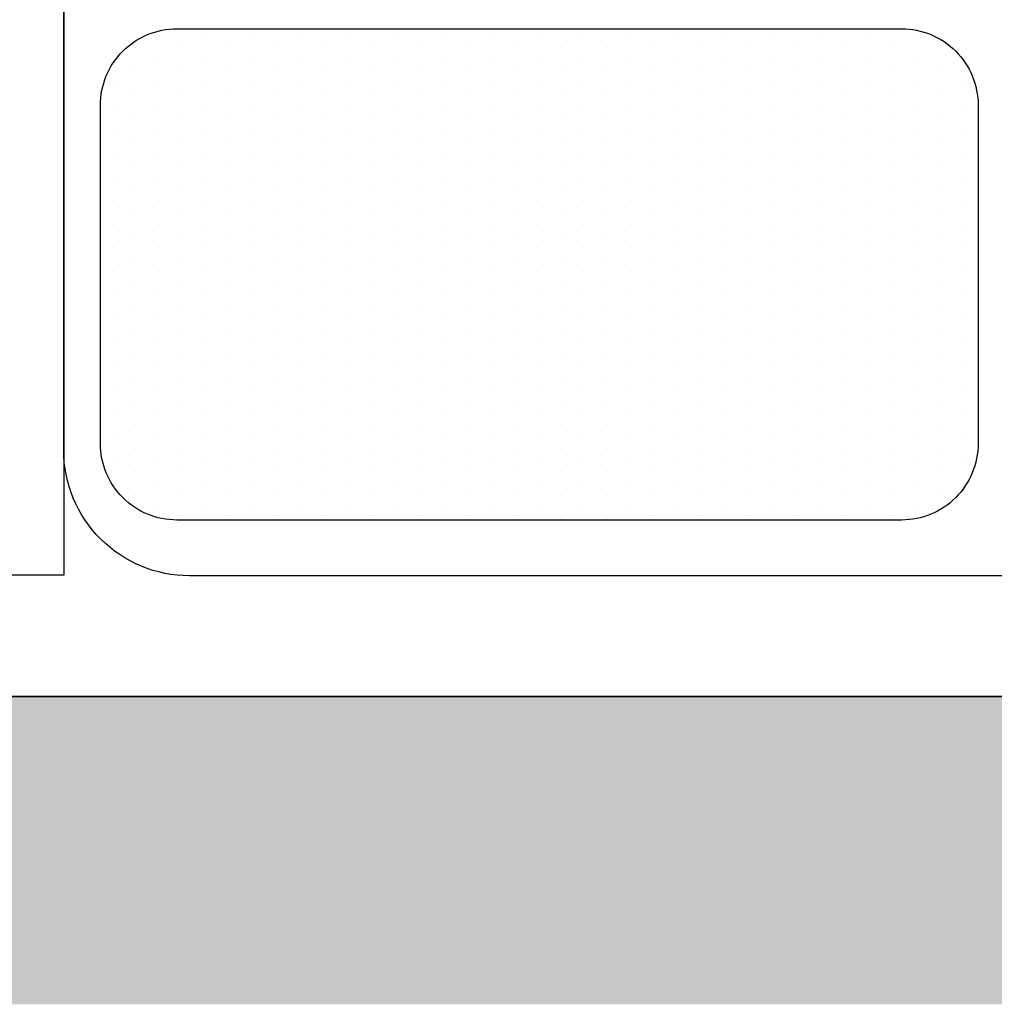
# Model space of a CAD drawing. Units: millimetres. Extents: x 2817 to 5038, y 1110 to 3565.
# Tile 3 of 21: x 2870 to 2898, y 1265 to 1294. Entities that reach past the tile are written whole.
import ezdxf

# ---------------------------------------------------------------- set-up
doc = ezdxf.new("R2010")
doc.units = ezdxf.units.MM
doc.layers.add('A-WALL', color=7, linetype='Continuous', lineweight=35)
doc.layers.add('FURNITURE', color=219, linetype='Continuous', lineweight=18)
doc.layers.add('A-WALL-PATT', color=51, linetype='Continuous', lineweight=13, true_color=0xf7f281)
doc.layers.add('BLOCK', color=6, linetype='Continuous')

# ---------------------------------------------------------------- blocks, each defined once
blk = doc.blocks.new('*X9')
at = {"color": 0}
for p, q in [((273.9375, 457.03125), (273.9375, 457.03125)), ((274.3125, 457.03125), (274.3125, 457.03125)), ((274.6875, 457.03125), (274.6875, 457.03125)), ((275.0625, 457.03125), (275.0625, 457.03125)), ((275.4375, 457.03125), (275.4375, 457.03125)), ((275.8125, 457.03125), (275.8125, 457.03125)), ((276.1875, 457.03125), (276.1875, 457.03125)), ((276.5625, 457.03125), (276.5625, 457.03125)), ((276.9375, 457.03125), (276.9375, 457.03125)), ((277.3125, 457.03125), (277.3125, 457.03125)), ((277.6875, 457.03125), (277.6875, 457.03125)), ((278.0625, 457.03125), (278.0625, 457.03125)), ((278.4375, 457.03125), (278.4375, 457.03125)), ((278.8125, 457.03125), (278.8125, 457.03125)), ((279.1875, 457.03125), (279.1875, 457.03125)), ((279.5625, 457.03125), (279.5625, 457.03125)), ((273.75, 456.9375), (273.75, 456.9375)), ((274.125, 456.9375), (274.125, 456.9375)), ((274.5, 456.9375), (274.5, 456.9375)), ((274.875, 456.9375), (274.875, 456.9375)), ((275.25, 456.9375), (275.25, 456.9375)), ((275.625, 456.9375), (275.625, 456.9375)), ((276, 456.9375), (276, 456.9375)), ((276.375, 456.9375), (276.375, 456.9375)), ((276.75, 456.9375), (276.75, 456.9375)), ((277.125, 456.9375), (277.125, 456.9375)), ((277.5, 456.9375), (277.5, 456.9375)), ((277.875, 456.9375), (277.875, 456.9375)), ((278.25, 456.9375), (278.25, 456.9375)), ((278.625, 456.9375), (278.625, 456.9375)), ((279, 456.9375), (279, 456.9375)), ((279.375, 456.9375), (279.375, 456.9375)), ((279.75, 456.9375), (279.75, 456.9375)), ((273.5625, 456.84375), (273.5625, 456.84375)), ((273.9375, 456.84375), (273.9375, 456.84375)), ((274.3125, 456.84375), (274.3125, 456.84375)), ((274.6875, 456.84375), (274.6875, 456.84375)), ((275.0625, 456.84375), (275.0625, 456.84375)), ((275.4375, 456.84375), (275.4375, 456.84375)), ((275.8125, 456.84375), (275.8125, 456.84375)), ((276.1875, 456.84375), (276.1875, 456.84375)), ((276.5625, 456.84375), (276.5625, 456.84375)), ((276.9375, 456.84375), (276.9375, 456.84375)), ((277.3125, 456.84375), (277.3125, 456.84375)), ((277.6875, 456.84375), (277.6875, 456.84375)), ((278.0625, 456.84375), (278.0625, 456.84375)), ((278.4375, 456.84375), (278.4375, 456.84375)), ((278.8125, 456.84375), (278.8125, 456.84375)), ((279.1875, 456.84375), (279.1875, 456.84375)), ((279.5625, 456.84375), (279.5625, 456.84375)), ((279.9375, 456.84375), (279.9375, 456.84375)), ((273.375, 456.75), (273.375, 456.75)), ((273.75, 456.75), (273.75, 456.75)), ((274.125, 456.75), (274.125, 456.75)), ((274.5, 456.75), (274.5, 456.75)), ((274.875, 456.75), (274.875, 456.75)), ((275.25, 456.75), (275.25, 456.75)), ((275.625, 456.75), (275.625, 456.75)), ((276, 456.75), (276, 456.75)), ((276.375, 456.75), (276.375, 456.75)), ((276.75, 456.75), (276.75, 456.75)), ((277.125, 456.75), (277.125, 456.75)), ((277.5, 456.75), (277.5, 456.75)), ((277.875, 456.75), (277.875, 456.75)), ((278.25, 456.75), (278.25, 456.75)), ((278.625, 456.75), (278.625, 456.75)), ((279, 456.75), (279, 456.75)), ((279.375, 456.75), (279.375, 456.75)), ((279.75, 456.75), (279.75, 456.75)), ((280.125, 456.75), (280.125, 456.75)), ((273.5625, 456.65625), (273.5625, 456.65625)), ((273.9375, 456.65625), (273.9375, 456.65625)), ((274.3125, 456.65625), (274.3125, 456.65625)), ((274.6875, 456.65625), (274.6875, 456.65625)), ((275.0625, 456.65625), (275.0625, 456.65625)), ((275.4375, 456.65625), (275.4375, 456.65625)), ((275.8125, 456.65625), (275.8125, 456.65625)), ((276.1875, 456.65625), (276.1875, 456.65625)), ((276.5625, 456.65625), (276.5625, 456.65625)), ((276.9375, 456.65625), (276.9375, 456.65625)), ((277.3125, 456.65625), (277.3125, 456.65625)), ((277.6875, 456.65625), (277.6875, 456.65625)), ((278.0625, 456.65625), (278.0625, 456.65625)), ((278.4375, 456.65625), (278.4375, 456.65625)), ((278.8125, 456.65625), (278.8125, 456.65625)), ((279.1875, 456.65625), (279.1875, 456.65625)), ((279.5625, 456.65625), (279.5625, 456.65625)), ((279.9375, 456.65625), (279.9375, 456.65625)), ((273.375, 456.5625), (273.375, 456.5625)), ((273.75, 456.5625), (273.75, 456.5625)), ((274.125, 456.5625), (274.125, 456.5625)), ((274.5, 456.5625), (274.5, 456.5625)), ((274.875, 456.5625), (274.875, 456.5625)), ((275.25, 456.5625), (275.25, 456.5625)), ((275.625, 456.5625), (275.625, 456.5625)), ((276, 456.5625), (276, 456.5625)), ((276.375, 456.5625), (276.375, 456.5625)), ((276.75, 456.5625), (276.75, 456.5625)), ((277.125, 456.5625), (277.125, 456.5625)), ((277.5, 456.5625), (277.5, 456.5625)), ((277.875, 456.5625), (277.875, 456.5625)), ((278.25, 456.5625), (278.25, 456.5625)), ((278.625, 456.5625), (278.625, 456.5625)), ((279, 456.5625), (279, 456.5625)), ((279.375, 456.5625), (279.375, 456.5625)), ((279.75, 456.5625), (279.75, 456.5625)), ((280.125, 456.5625), (280.125, 456.5625)), ((273.5625, 456.46875), (273.5625, 456.46875)), ((273.9375, 456.46875), (273.9375, 456.46875)), ((274.3125, 456.46875), (274.3125, 456.46875)), ((274.6875, 456.46875), (274.6875, 456.46875)), ((275.0625, 456.46875), (275.0625, 456.46875)), ((275.4375, 456.46875), (275.4375, 456.46875)), ((275.8125, 456.46875), (275.8125, 456.46875)), ((276.1875, 456.46875), (276.1875, 456.46875)), ((276.5625, 456.46875), (276.5625, 456.46875)), ((276.9375, 456.46875), (276.9375, 456.46875)), ((277.3125, 456.46875), (277.3125, 456.46875)), ((277.6875, 456.46875), (277.6875, 456.46875)), ((278.0625, 456.46875), (278.0625, 456.46875)), ((278.4375, 456.46875), (278.4375, 456.46875)), ((278.8125, 456.46875), (278.8125, 456.46875)), ((279.1875, 456.46875), (279.1875, 456.46875)), ((279.5625, 456.46875), (279.5625, 456.46875)), ((279.9375, 456.46875), (279.9375, 456.46875)), ((273.375, 456.375), (273.375, 456.375)), ((273.75, 456.375), (273.75, 456.375)), ((274.125, 456.375), (274.125, 456.375)), ((274.5, 456.375), (274.5, 456.375)), ((274.875, 456.375), (274.875, 456.375)), ((275.25, 456.375), (275.25, 456.375)), ((275.625, 456.375), (275.625, 456.375)), ((276, 456.375), (276, 456.375)), ((276.375, 456.375), (276.375, 456.375)), ((276.75, 456.375), (276.75, 456.375)), ((277.125, 456.375), (277.125, 456.375)), ((277.5, 456.375), (277.5, 456.375)), ((277.875, 456.375), (277.875, 456.375)), ((278.25, 456.375), (278.25, 456.375)), ((278.625, 456.375), (278.625, 456.375)), ((279, 456.375), (279, 456.375)), ((279.375, 456.375), (279.375, 456.375)), ((279.75, 456.375), (279.75, 456.375)), ((280.125, 456.375), (280.125, 456.375)), ((273.5625, 456.28125), (273.5625, 456.28125)), ((273.9375, 456.28125), (273.9375, 456.28125)), ((274.3125, 456.28125), (274.3125, 456.28125)), ((274.6875, 456.28125), (274.6875, 456.28125)), ((275.0625, 456.28125), (275.0625, 456.28125)), ((275.4375, 456.28125), (275.4375, 456.28125)), ((275.8125, 456.28125), (275.8125, 456.28125)), ((276.1875, 456.28125), (276.1875, 456.28125)), ((276.5625, 456.28125), (276.5625, 456.28125)), ((276.9375, 456.28125), (276.9375, 456.28125)), ((277.3125, 456.28125), (277.3125, 456.28125)), ((277.6875, 456.28125), (277.6875, 456.28125)), ((278.0625, 456.28125), (278.0625, 456.28125)), ((278.4375, 456.28125), (278.4375, 456.28125)), ((278.8125, 456.28125), (278.8125, 456.28125)), ((279.1875, 456.28125), (279.1875, 456.28125)), ((279.5625, 456.28125), (279.5625, 456.28125)), ((279.9375, 456.28125), (279.9375, 456.28125)), ((273.375, 456.1875), (273.375, 456.1875)), ((273.75, 456.1875), (273.75, 456.1875)), ((274.125, 456.1875), (274.125, 456.1875)), ((274.5, 456.1875), (274.5, 456.1875)), ((274.875, 456.1875), (274.875, 456.1875)), ((275.25, 456.1875), (275.25, 456.1875)), ((275.625, 456.1875), (275.625, 456.1875)), ((276, 456.1875), (276, 456.1875)), ((276.375, 456.1875), (276.375, 456.1875)), ((276.75, 456.1875), (276.75, 456.1875)), ((277.125, 456.1875), (277.125, 456.1875)), ((277.5, 456.1875), (277.5, 456.1875)), ((277.875, 456.1875), (277.875, 456.1875)), ((278.25, 456.1875), (278.25, 456.1875)), ((278.625, 456.1875), (278.625, 456.1875)), ((279, 456.1875), (279, 456.1875)), ((279.375, 456.1875), (279.375, 456.1875)), ((279.75, 456.1875), (279.75, 456.1875)), ((280.125, 456.1875), (280.125, 456.1875)), ((273.5625, 456.09375), (273.5625, 456.09375)), ((273.9375, 456.09375), (273.9375, 456.09375)), ((274.3125, 456.09375), (274.3125, 456.09375)), ((274.6875, 456.09375), (274.6875, 456.09375)), ((275.0625, 456.09375), (275.0625, 456.09375)), ((275.4375, 456.09375), (275.4375, 456.09375)), ((275.8125, 456.09375), (275.8125, 456.09375)), ((276.1875, 456.09375), (276.1875, 456.09375)), ((276.5625, 456.09375), (276.5625, 456.09375)), ((276.9375, 456.09375), (276.9375, 456.09375)), ((277.3125, 456.09375), (277.3125, 456.09375)), ((277.6875, 456.09375), (277.6875, 456.09375)), ((278.0625, 456.09375), (278.0625, 456.09375)), ((278.4375, 456.09375), (278.4375, 456.09375)), ((278.8125, 456.09375), (278.8125, 456.09375)), ((279.1875, 456.09375), (279.1875, 456.09375)), ((279.5625, 456.09375), (279.5625, 456.09375)), ((279.9375, 456.09375), (279.9375, 456.09375)), ((273.375, 456), (273.375, 456)), ((273.75, 456), (273.75, 456)), ((274.125, 456), (274.125, 456)), ((274.5, 456), (274.5, 456)), ((274.875, 456), (274.875, 456)), ((275.25, 456), (275.25, 456)), ((275.625, 456), (275.625, 456)), ((276, 456), (276, 456)), ((276.375, 456), (276.375, 456)), ((276.75, 456), (276.75, 456)), ((277.125, 456), (277.125, 456)), ((277.5, 456), (277.5, 456)), ((277.875, 456), (277.875, 456)), ((278.25, 456), (278.25, 456)), ((278.625, 456), (278.625, 456)), ((279, 456), (279, 456)), ((279.375, 456), (279.375, 456)), ((279.75, 456), (279.75, 456)), ((280.125, 456), (280.125, 456)), ((273.5625, 455.90625), (273.5625, 455.90625)), ((273.9375, 455.90625), (273.9375, 455.90625)), ((274.3125, 455.90625), (274.3125, 455.90625)), ((274.6875, 455.90625), (274.6875, 455.90625)), ((275.0625, 455.90625), (275.0625, 455.90625)), ((275.4375, 455.90625), (275.4375, 455.90625)), ((275.8125, 455.90625), (275.8125, 455.90625)), ((276.1875, 455.90625), (276.1875, 455.90625)), ((276.5625, 455.90625), (276.5625, 455.90625)), ((276.9375, 455.90625), (276.9375, 455.90625)), ((277.3125, 455.90625), (277.3125, 455.90625)), ((277.6875, 455.90625), (277.6875, 455.90625)), ((278.0625, 455.90625), (278.0625, 455.90625)), ((278.4375, 455.90625), (278.4375, 455.90625)), ((278.8125, 455.90625), (278.8125, 455.90625)), ((279.1875, 455.90625), (279.1875, 455.90625)), ((279.5625, 455.90625), (279.5625, 455.90625)), ((279.9375, 455.90625), (279.9375, 455.90625)), ((273.375, 455.8125), (273.375, 455.8125)), ((273.75, 455.8125), (273.75, 455.8125)), ((274.125, 455.8125), (274.125, 455.8125)), ((274.5, 455.8125), (274.5, 455.8125)), ((274.875, 455.8125), (274.875, 455.8125)), ((275.25, 455.8125), (275.25, 455.8125)), ((275.625, 455.8125), (275.625, 455.8125)), ((276, 455.8125), (276, 455.8125)), ((276.375, 455.8125), (276.375, 455.8125)), ((276.75, 455.8125), (276.75, 455.8125)), ((277.125, 455.8125), (277.125, 455.8125)), ((277.5, 455.8125), (277.5, 455.8125)), ((277.875, 455.8125), (277.875, 455.8125)), ((278.25, 455.8125), (278.25, 455.8125)), ((278.625, 455.8125), (278.625, 455.8125)), ((279, 455.8125), (279, 455.8125)), ((279.375, 455.8125), (279.375, 455.8125)), ((279.75, 455.8125), (279.75, 455.8125)), ((280.125, 455.8125), (280.125, 455.8125)), ((273.5625, 455.71875), (273.5625, 455.71875)), ((273.9375, 455.71875), (273.9375, 455.71875)), ((274.3125, 455.71875), (274.3125, 455.71875)), ((274.6875, 455.71875), (274.6875, 455.71875)), ((275.0625, 455.71875), (275.0625, 455.71875)), ((275.4375, 455.71875), (275.4375, 455.71875)), ((275.8125, 455.71875), (275.8125, 455.71875)), ((276.1875, 455.71875), (276.1875, 455.71875)), ((276.5625, 455.71875), (276.5625, 455.71875)), ((276.9375, 455.71875), (276.9375, 455.71875)), ((277.3125, 455.71875), (277.3125, 455.71875)), ((277.6875, 455.71875), (277.6875, 455.71875)), ((278.0625, 455.71875), (278.0625, 455.71875)), ((278.4375, 455.71875), (278.4375, 455.71875)), ((278.8125, 455.71875), (278.8125, 455.71875)), ((279.1875, 455.71875), (279.1875, 455.71875)), ((279.5625, 455.71875), (279.5625, 455.71875)), ((279.9375, 455.71875), (279.9375, 455.71875)), ((273.375, 455.625), (273.375, 455.625)), ((273.75, 455.625), (273.75, 455.625)), ((274.125, 455.625), (274.125, 455.625)), ((274.5, 455.625), (274.5, 455.625)), ((274.875, 455.625), (274.875, 455.625)), ((275.25, 455.625), (275.25, 455.625)), ((275.625, 455.625), (275.625, 455.625)), ((276, 455.625), (276, 455.625)), ((276.375, 455.625), (276.375, 455.625)), ((276.75, 455.625), (276.75, 455.625)), ((277.125, 455.625), (277.125, 455.625)), ((277.5, 455.625), (277.5, 455.625)), ((277.875, 455.625), (277.875, 455.625)), ((278.25, 455.625), (278.25, 455.625)), ((278.625, 455.625), (278.625, 455.625)), ((279, 455.625), (279, 455.625)), ((279.375, 455.625), (279.375, 455.625)), ((279.75, 455.625), (279.75, 455.625)), ((280.125, 455.625), (280.125, 455.625)), ((273.5625, 455.53125), (273.5625, 455.53125)), ((273.9375, 455.53125), (273.9375, 455.53125)), ((274.3125, 455.53125), (274.3125, 455.53125)), ((274.6875, 455.53125), (274.6875, 455.53125)), ((275.0625, 455.53125), (275.0625, 455.53125)), ((275.4375, 455.53125), (275.4375, 455.53125)), ((275.8125, 455.53125), (275.8125, 455.53125)), ((276.1875, 455.53125), (276.1875, 455.53125)), ((276.5625, 455.53125), (276.5625, 455.53125)), ((276.9375, 455.53125), (276.9375, 455.53125)), ((277.3125, 455.53125), (277.3125, 455.53125)), ((277.6875, 455.53125), (277.6875, 455.53125)), ((278.0625, 455.53125), (278.0625, 455.53125)), ((278.4375, 455.53125), (278.4375, 455.53125)), ((278.8125, 455.53125), (278.8125, 455.53125)), ((279.1875, 455.53125), (279.1875, 455.53125)), ((279.5625, 455.53125), (279.5625, 455.53125)), ((279.9375, 455.53125), (279.9375, 455.53125)), ((273.375, 455.4375), (273.375, 455.4375)), ((273.75, 455.4375), (273.75, 455.4375)), ((274.125, 455.4375), (274.125, 455.4375)), ((274.5, 455.4375), (274.5, 455.4375)), ((274.875, 455.4375), (274.875, 455.4375)), ((275.25, 455.4375), (275.25, 455.4375)), ((275.625, 455.4375), (275.625, 455.4375)), ((276, 455.4375), (276, 455.4375)), ((276.375, 455.4375), (276.375, 455.4375)), ((276.75, 455.4375), (276.75, 455.4375)), ((277.125, 455.4375), (277.125, 455.4375)), ((277.5, 455.4375), (277.5, 455.4375)), ((277.875, 455.4375), (277.875, 455.4375)), ((278.25, 455.4375), (278.25, 455.4375)), ((278.625, 455.4375), (278.625, 455.4375)), ((279, 455.4375), (279, 455.4375)), ((279.375, 455.4375), (279.375, 455.4375)), ((279.75, 455.4375), (279.75, 455.4375)), ((280.125, 455.4375), (280.125, 455.4375)), ((273.5625, 455.34375), (273.5625, 455.34375)), ((273.9375, 455.34375), (273.9375, 455.34375)), ((274.3125, 455.34375), (274.3125, 455.34375)), ((274.6875, 455.34375), (274.6875, 455.34375)), ((275.0625, 455.34375), (275.0625, 455.34375)), ((275.4375, 455.34375), (275.4375, 455.34375)), ((275.8125, 455.34375), (275.8125, 455.34375)), ((276.1875, 455.34375), (276.1875, 455.34375)), ((276.5625, 455.34375), (276.5625, 455.34375)), ((276.9375, 455.34375), (276.9375, 455.34375)), ((277.3125, 455.34375), (277.3125, 455.34375)), ((277.6875, 455.34375), (277.6875, 455.34375)), ((278.0625, 455.34375), (278.0625, 455.34375)), ((278.4375, 455.34375), (278.4375, 455.34375)), ((278.8125, 455.34375), (278.8125, 455.34375)), ((279.1875, 455.34375), (279.1875, 455.34375)), ((279.5625, 455.34375), (279.5625, 455.34375)), ((279.9375, 455.34375), (279.9375, 455.34375)), ((273.375, 455.25), (273.375, 455.25)), ((273.75, 455.25), (273.75, 455.25)), ((274.125, 455.25), (274.125, 455.25)), ((274.5, 455.25), (274.5, 455.25)), ((274.875, 455.25), (274.875, 455.25)), ((275.25, 455.25), (275.25, 455.25)), ((275.625, 455.25), (275.625, 455.25)), ((276, 455.25), (276, 455.25)), ((276.375, 455.25), (276.375, 455.25)), ((276.75, 455.25), (276.75, 455.25)), ((277.125, 455.25), (277.125, 455.25)), ((277.5, 455.25), (277.5, 455.25)), ((277.875, 455.25), (277.875, 455.25)), ((278.25, 455.25), (278.25, 455.25)), ((278.625, 455.25), (278.625, 455.25)), ((279, 455.25), (279, 455.25)), ((279.375, 455.25), (279.375, 455.25)), ((279.75, 455.25), (279.75, 455.25)), ((280.125, 455.25), (280.125, 455.25)), ((273.5625, 455.15625), (273.5625, 455.15625)), ((273.9375, 455.15625), (273.9375, 455.15625)), ((274.3125, 455.15625), (274.3125, 455.15625)), ((274.6875, 455.15625), (274.6875, 455.15625)), ((275.0625, 455.15625), (275.0625, 455.15625)), ((275.4375, 455.15625), (275.4375, 455.15625)), ((275.8125, 455.15625), (275.8125, 455.15625)), ((276.1875, 455.15625), (276.1875, 455.15625)), ((276.5625, 455.15625), (276.5625, 455.15625)), ((276.9375, 455.15625), (276.9375, 455.15625)), ((277.3125, 455.15625), (277.3125, 455.15625)), ((277.6875, 455.15625), (277.6875, 455.15625)), ((278.0625, 455.15625), (278.0625, 455.15625)), ((278.4375, 455.15625), (278.4375, 455.15625)), ((278.8125, 455.15625), (278.8125, 455.15625)), ((279.1875, 455.15625), (279.1875, 455.15625)), ((279.5625, 455.15625), (279.5625, 455.15625)), ((279.9375, 455.15625), (279.9375, 455.15625)), ((273.375, 455.0625), (273.375, 455.0625)), ((273.75, 455.0625), (273.75, 455.0625)), ((274.125, 455.0625), (274.125, 455.0625)), ((274.5, 455.0625), (274.5, 455.0625)), ((274.875, 455.0625), (274.875, 455.0625)), ((275.25, 455.0625), (275.25, 455.0625)), ((275.625, 455.0625), (275.625, 455.0625)), ((276, 455.0625), (276, 455.0625)), ((276.375, 455.0625), (276.375, 455.0625)), ((276.75, 455.0625), (276.75, 455.0625)), ((277.125, 455.0625), (277.125, 455.0625)), ((277.5, 455.0625), (277.5, 455.0625)), ((277.875, 455.0625), (277.875, 455.0625)), ((278.25, 455.0625), (278.25, 455.0625)), ((278.625, 455.0625), (278.625, 455.0625)), ((279, 455.0625), (279, 455.0625)), ((279.375, 455.0625), (279.375, 455.0625)), ((279.75, 455.0625), (279.75, 455.0625)), ((280.125, 455.0625), (280.125, 455.0625)), ((273.5625, 454.96875), (273.5625, 454.96875)), ((273.9375, 454.96875), (273.9375, 454.96875)), ((274.3125, 454.96875), (274.3125, 454.96875)), ((274.6875, 454.96875), (274.6875, 454.96875)), ((275.0625, 454.96875), (275.0625, 454.96875)), ((275.4375, 454.96875), (275.4375, 454.96875)), ((275.8125, 454.96875), (275.8125, 454.96875)), ((276.1875, 454.96875), (276.1875, 454.96875)), ((276.5625, 454.96875), (276.5625, 454.96875)), ((276.9375, 454.96875), (276.9375, 454.96875)), ((277.3125, 454.96875), (277.3125, 454.96875)), ((277.6875, 454.96875), (277.6875, 454.96875)), ((278.0625, 454.96875), (278.0625, 454.96875)), ((278.4375, 454.96875), (278.4375, 454.96875)), ((278.8125, 454.96875), (278.8125, 454.96875)), ((279.1875, 454.96875), (279.1875, 454.96875)), ((279.5625, 454.96875), (279.5625, 454.96875)), ((279.9375, 454.96875), (279.9375, 454.96875)), ((273.375, 454.875), (273.375, 454.875)), ((273.75, 454.875), (273.75, 454.875)), ((274.125, 454.875), (274.125, 454.875)), ((274.5, 454.875), (274.5, 454.875)), ((274.875, 454.875), (274.875, 454.875)), ((275.25, 454.875), (275.25, 454.875)), ((275.625, 454.875), (275.625, 454.875)), ((276, 454.875), (276, 454.875)), ((276.375, 454.875), (276.375, 454.875)), ((276.75, 454.875), (276.75, 454.875)), ((277.125, 454.875), (277.125, 454.875)), ((277.5, 454.875), (277.5, 454.875)), ((277.875, 454.875), (277.875, 454.875)), ((278.25, 454.875), (278.25, 454.875)), ((278.625, 454.875), (278.625, 454.875)), ((279, 454.875), (279, 454.875)), ((279.375, 454.875), (279.375, 454.875)), ((279.75, 454.875), (279.75, 454.875)), ((280.125, 454.875), (280.125, 454.875)), ((273.5625, 454.78125), (273.5625, 454.78125)), ((273.9375, 454.78125), (273.9375, 454.78125)), ((274.3125, 454.78125), (274.3125, 454.78125)), ((274.6875, 454.78125), (274.6875, 454.78125)), ((275.0625, 454.78125), (275.0625, 454.78125)), ((275.4375, 454.78125), (275.4375, 454.78125)), ((275.8125, 454.78125), (275.8125, 454.78125)), ((276.1875, 454.78125), (276.1875, 454.78125)), ((276.5625, 454.78125), (276.5625, 454.78125)), ((276.9375, 454.78125), (276.9375, 454.78125)), ((277.3125, 454.78125), (277.3125, 454.78125)), ((277.6875, 454.78125), (277.6875, 454.78125)), ((278.0625, 454.78125), (278.0625, 454.78125)), ((278.4375, 454.78125), (278.4375, 454.78125)), ((278.8125, 454.78125), (278.8125, 454.78125)), ((279.1875, 454.78125), (279.1875, 454.78125)), ((279.5625, 454.78125), (279.5625, 454.78125)), ((279.9375, 454.78125), (279.9375, 454.78125)), ((273.375, 454.6875), (273.375, 454.6875)), ((273.75, 454.6875), (273.75, 454.6875)), ((274.125, 454.6875), (274.125, 454.6875)), ((274.5, 454.6875), (274.5, 454.6875)), ((274.875, 454.6875), (274.875, 454.6875)), ((275.25, 454.6875), (275.25, 454.6875)), ((275.625, 454.6875), (275.625, 454.6875)), ((276, 454.6875), (276, 454.6875)), ((276.375, 454.6875), (276.375, 454.6875)), ((276.75, 454.6875), (276.75, 454.6875)), ((277.125, 454.6875), (277.125, 454.6875)), ((277.5, 454.6875), (277.5, 454.6875)), ((277.875, 454.6875), (277.875, 454.6875)), ((278.25, 454.6875), (278.25, 454.6875)), ((278.625, 454.6875), (278.625, 454.6875)), ((279, 454.6875), (279, 454.6875)), ((279.375, 454.6875), (279.375, 454.6875)), ((279.75, 454.6875), (279.75, 454.6875)), ((280.125, 454.6875), (280.125, 454.6875)), ((273.5625, 454.59375), (273.5625, 454.59375)), ((273.9375, 454.59375), (273.9375, 454.59375)), ((274.3125, 454.59375), (274.3125, 454.59375)), ((274.6875, 454.59375), (274.6875, 454.59375)), ((275.0625, 454.59375), (275.0625, 454.59375)), ((275.4375, 454.59375), (275.4375, 454.59375)), ((275.8125, 454.59375), (275.8125, 454.59375)), ((276.1875, 454.59375), (276.1875, 454.59375)), ((276.5625, 454.59375), (276.5625, 454.59375)), ((276.9375, 454.59375), (276.9375, 454.59375)), ((277.3125, 454.59375), (277.3125, 454.59375)), ((277.6875, 454.59375), (277.6875, 454.59375)), ((278.0625, 454.59375), (278.0625, 454.59375)), ((278.4375, 454.59375), (278.4375, 454.59375)), ((278.8125, 454.59375), (278.8125, 454.59375)), ((279.1875, 454.59375), (279.1875, 454.59375)), ((279.5625, 454.59375), (279.5625, 454.59375)), ((279.9375, 454.59375), (279.9375, 454.59375)), ((273.375, 454.5), (273.375, 454.5)), ((273.75, 454.5), (273.75, 454.5)), ((274.125, 454.5), (274.125, 454.5)), ((274.5, 454.5), (274.5, 454.5)), ((274.875, 454.5), (274.875, 454.5)), ((275.25, 454.5), (275.25, 454.5)), ((275.625, 454.5), (275.625, 454.5)), ((276, 454.5), (276, 454.5)), ((276.375, 454.5), (276.375, 454.5)), ((276.75, 454.5), (276.75, 454.5)), ((277.125, 454.5), (277.125, 454.5)), ((277.5, 454.5), (277.5, 454.5)), ((277.875, 454.5), (277.875, 454.5)), ((278.25, 454.5), (278.25, 454.5)), ((278.625, 454.5), (278.625, 454.5)), ((279, 454.5), (279, 454.5)), ((279.375, 454.5), (279.375, 454.5)), ((279.75, 454.5), (279.75, 454.5)), ((280.125, 454.5), (280.125, 454.5)), ((273.5625, 454.40625), (273.5625, 454.40625)), ((273.9375, 454.40625), (273.9375, 454.40625)), ((274.3125, 454.40625), (274.3125, 454.40625)), ((274.6875, 454.40625), (274.6875, 454.40625)), ((275.0625, 454.40625), (275.0625, 454.40625)), ((275.4375, 454.40625), (275.4375, 454.40625)), ((275.8125, 454.40625), (275.8125, 454.40625)), ((276.1875, 454.40625), (276.1875, 454.40625)), ((276.5625, 454.40625), (276.5625, 454.40625)), ((276.9375, 454.40625), (276.9375, 454.40625)), ((277.3125, 454.40625), (277.3125, 454.40625)), ((277.6875, 454.40625), (277.6875, 454.40625)), ((278.0625, 454.40625), (278.0625, 454.40625)), ((278.4375, 454.40625), (278.4375, 454.40625)), ((278.8125, 454.40625), (278.8125, 454.40625)), ((279.1875, 454.40625), (279.1875, 454.40625)), ((279.5625, 454.40625), (279.5625, 454.40625)), ((279.9375, 454.40625), (279.9375, 454.40625)), ((273.375, 454.3125), (273.375, 454.3125)), ((273.75, 454.3125), (273.75, 454.3125)), ((274.125, 454.3125), (274.125, 454.3125)), ((274.5, 454.3125), (274.5, 454.3125)), ((274.875, 454.3125), (274.875, 454.3125)), ((275.25, 454.3125), (275.25, 454.3125)), ((275.625, 454.3125), (275.625, 454.3125)), ((276, 454.3125), (276, 454.3125)), ((276.375, 454.3125), (276.375, 454.3125)), ((276.75, 454.3125), (276.75, 454.3125)), ((277.125, 454.3125), (277.125, 454.3125)), ((277.5, 454.3125), (277.5, 454.3125)), ((277.875, 454.3125), (277.875, 454.3125)), ((278.25, 454.3125), (278.25, 454.3125)), ((278.625, 454.3125), (278.625, 454.3125)), ((279, 454.3125), (279, 454.3125)), ((279.375, 454.3125), (279.375, 454.3125)), ((279.75, 454.3125), (279.75, 454.3125)), ((280.125, 454.3125), (280.125, 454.3125)), ((273.5625, 454.21875), (273.5625, 454.21875)), ((273.9375, 454.21875), (273.9375, 454.21875)), ((274.3125, 454.21875), (274.3125, 454.21875)), ((274.6875, 454.21875), (274.6875, 454.21875)), ((275.0625, 454.21875), (275.0625, 454.21875)), ((275.4375, 454.21875), (275.4375, 454.21875)), ((275.8125, 454.21875), (275.8125, 454.21875)), ((276.1875, 454.21875), (276.1875, 454.21875)), ((276.5625, 454.21875), (276.5625, 454.21875)), ((276.9375, 454.21875), (276.9375, 454.21875)), ((277.3125, 454.21875), (277.3125, 454.21875)), ((277.6875, 454.21875), (277.6875, 454.21875)), ((278.0625, 454.21875), (278.0625, 454.21875)), ((278.4375, 454.21875), (278.4375, 454.21875)), ((278.8125, 454.21875), (278.8125, 454.21875)), ((279.1875, 454.21875), (279.1875, 454.21875)), ((279.5625, 454.21875), (279.5625, 454.21875)), ((279.9375, 454.21875), (279.9375, 454.21875)), ((273.375, 454.125), (273.375, 454.125)), ((273.75, 454.125), (273.75, 454.125)), ((274.125, 454.125), (274.125, 454.125)), ((274.5, 454.125), (274.5, 454.125)), ((274.875, 454.125), (274.875, 454.125)), ((275.25, 454.125), (275.25, 454.125)), ((275.625, 454.125), (275.625, 454.125)), ((276, 454.125), (276, 454.125)), ((276.375, 454.125), (276.375, 454.125)), ((276.75, 454.125), (276.75, 454.125)), ((277.125, 454.125), (277.125, 454.125)), ((277.5, 454.125), (277.5, 454.125)), ((277.875, 454.125), (277.875, 454.125)), ((278.25, 454.125), (278.25, 454.125)), ((278.625, 454.125), (278.625, 454.125)), ((279, 454.125), (279, 454.125)), ((279.375, 454.125), (279.375, 454.125)), ((279.75, 454.125), (279.75, 454.125)), ((280.125, 454.125), (280.125, 454.125)), ((273.5625, 454.03125), (273.5625, 454.03125)), ((273.9375, 454.03125), (273.9375, 454.03125)), ((274.3125, 454.03125), (274.3125, 454.03125)), ((274.6875, 454.03125), (274.6875, 454.03125)), ((275.0625, 454.03125), (275.0625, 454.03125)), ((275.4375, 454.03125), (275.4375, 454.03125)), ((275.8125, 454.03125), (275.8125, 454.03125)), ((276.1875, 454.03125), (276.1875, 454.03125)), ((276.5625, 454.03125), (276.5625, 454.03125)), ((276.9375, 454.03125), (276.9375, 454.03125)), ((277.3125, 454.03125), (277.3125, 454.03125)), ((277.6875, 454.03125), (277.6875, 454.03125)), ((278.0625, 454.03125), (278.0625, 454.03125)), ((278.4375, 454.03125), (278.4375, 454.03125)), ((278.8125, 454.03125), (278.8125, 454.03125)), ((279.1875, 454.03125), (279.1875, 454.03125)), ((279.5625, 454.03125), (279.5625, 454.03125)), ((279.9375, 454.03125), (279.9375, 454.03125)), ((273.375, 453.9375), (273.375, 453.9375)), ((273.75, 453.9375), (273.75, 453.9375)), ((274.125, 453.9375), (274.125, 453.9375)), ((274.5, 453.9375), (274.5, 453.9375)), ((274.875, 453.9375), (274.875, 453.9375)), ((275.25, 453.9375), (275.25, 453.9375)), ((275.625, 453.9375), (275.625, 453.9375)), ((276, 453.9375), (276, 453.9375)), ((276.375, 453.9375), (276.375, 453.9375)), ((276.75, 453.9375), (276.75, 453.9375)), ((277.125, 453.9375), (277.125, 453.9375)), ((277.5, 453.9375), (277.5, 453.9375)), ((277.875, 453.9375), (277.875, 453.9375)), ((278.25, 453.9375), (278.25, 453.9375)), ((278.625, 453.9375), (278.625, 453.9375)), ((279, 453.9375), (279, 453.9375)), ((279.375, 453.9375), (279.375, 453.9375)), ((279.75, 453.9375), (279.75, 453.9375)), ((280.125, 453.9375), (280.125, 453.9375)), ((273.5625, 453.84375), (273.5625, 453.84375)), ((273.9375, 453.84375), (273.9375, 453.84375)), ((274.3125, 453.84375), (274.3125, 453.84375)), ((274.6875, 453.84375), (274.6875, 453.84375)), ((275.0625, 453.84375), (275.0625, 453.84375)), ((275.4375, 453.84375), (275.4375, 453.84375)), ((275.8125, 453.84375), (275.8125, 453.84375)), ((276.1875, 453.84375), (276.1875, 453.84375)), ((276.5625, 453.84375), (276.5625, 453.84375)), ((276.9375, 453.84375), (276.9375, 453.84375)), ((277.3125, 453.84375), (277.3125, 453.84375)), ((277.6875, 453.84375), (277.6875, 453.84375)), ((278.0625, 453.84375), (278.0625, 453.84375)), ((278.4375, 453.84375), (278.4375, 453.84375)), ((278.8125, 453.84375), (278.8125, 453.84375)), ((279.1875, 453.84375), (279.1875, 453.84375)), ((279.5625, 453.84375), (279.5625, 453.84375)), ((279.9375, 453.84375), (279.9375, 453.84375)), ((273.375, 453.75), (273.375, 453.75)), ((273.75, 453.75), (273.75, 453.75)), ((274.125, 453.75), (274.125, 453.75)), ((274.5, 453.75), (274.5, 453.75)), ((274.875, 453.75), (274.875, 453.75)), ((275.25, 453.75), (275.25, 453.75)), ((275.625, 453.75), (275.625, 453.75)), ((276, 453.75), (276, 453.75)), ((276.375, 453.75), (276.375, 453.75)), ((276.75, 453.75), (276.75, 453.75)), ((277.125, 453.75), (277.125, 453.75)), ((277.5, 453.75), (277.5, 453.75)), ((277.875, 453.75), (277.875, 453.75)), ((278.25, 453.75), (278.25, 453.75)), ((278.625, 453.75), (278.625, 453.75)), ((279, 453.75), (279, 453.75)), ((279.375, 453.75), (279.375, 453.75)), ((279.75, 453.75), (279.75, 453.75)), ((280.125, 453.75), (280.125, 453.75)), ((273.5625, 453.65625), (273.5625, 453.65625)), ((273.9375, 453.65625), (273.9375, 453.65625)), ((274.3125, 453.65625), (274.3125, 453.65625)), ((274.6875, 453.65625), (274.6875, 453.65625)), ((275.0625, 453.65625), (275.0625, 453.65625)), ((275.4375, 453.65625), (275.4375, 453.65625)), ((275.8125, 453.65625), (275.8125, 453.65625)), ((276.1875, 453.65625), (276.1875, 453.65625)), ((276.5625, 453.65625), (276.5625, 453.65625)), ((276.9375, 453.65625), (276.9375, 453.65625)), ((277.3125, 453.65625), (277.3125, 453.65625)), ((277.6875, 453.65625), (277.6875, 453.65625)), ((278.0625, 453.65625), (278.0625, 453.65625)), ((278.4375, 453.65625), (278.4375, 453.65625)), ((278.8125, 453.65625), (278.8125, 453.65625)), ((279.1875, 453.65625), (279.1875, 453.65625)), ((279.5625, 453.65625), (279.5625, 453.65625)), ((279.9375, 453.65625), (279.9375, 453.65625)), ((273.375, 453.5625), (273.375, 453.5625)), ((273.75, 453.5625), (273.75, 453.5625)), ((274.125, 453.5625), (274.125, 453.5625)), ((274.5, 453.5625), (274.5, 453.5625)), ((274.875, 453.5625), (274.875, 453.5625)), ((275.25, 453.5625), (275.25, 453.5625)), ((275.625, 453.5625), (275.625, 453.5625)), ((276, 453.5625), (276, 453.5625)), ((276.375, 453.5625), (276.375, 453.5625)), ((276.75, 453.5625), (276.75, 453.5625)), ((277.125, 453.5625), (277.125, 453.5625)), ((277.5, 453.5625), (277.5, 453.5625)), ((277.875, 453.5625), (277.875, 453.5625)), ((278.25, 453.5625), (278.25, 453.5625)), ((278.625, 453.5625), (278.625, 453.5625)), ((279, 453.5625), (279, 453.5625)), ((279.375, 453.5625), (279.375, 453.5625)), ((279.75, 453.5625), (279.75, 453.5625)), ((280.125, 453.5625), (280.125, 453.5625)), ((273.5625, 453.46875), (273.5625, 453.46875)), ((273.9375, 453.46875), (273.9375, 453.46875)), ((274.3125, 453.46875), (274.3125, 453.46875)), ((274.6875, 453.46875), (274.6875, 453.46875)), ((275.0625, 453.46875), (275.0625, 453.46875)), ((275.4375, 453.46875), (275.4375, 453.46875)), ((275.8125, 453.46875), (275.8125, 453.46875)), ((276.1875, 453.46875), (276.1875, 453.46875)), ((276.5625, 453.46875), (276.5625, 453.46875)), ((276.9375, 453.46875), (276.9375, 453.46875)), ((277.3125, 453.46875), (277.3125, 453.46875)), ((277.6875, 453.46875), (277.6875, 453.46875)), ((278.0625, 453.46875), (278.0625, 453.46875)), ((278.4375, 453.46875), (278.4375, 453.46875)), ((278.8125, 453.46875), (278.8125, 453.46875)), ((279.1875, 453.46875), (279.1875, 453.46875)), ((279.5625, 453.46875), (279.5625, 453.46875)), ((279.9375, 453.46875), (279.9375, 453.46875)), ((273.375, 453.375), (273.375, 453.375)), ((273.75, 453.375), (273.75, 453.375)), ((274.125, 453.375), (274.125, 453.375)), ((274.5, 453.375), (274.5, 453.375)), ((274.875, 453.375), (274.875, 453.375)), ((275.25, 453.375), (275.25, 453.375)), ((275.625, 453.375), (275.625, 453.375)), ((276, 453.375), (276, 453.375)), ((276.375, 453.375), (276.375, 453.375)), ((276.75, 453.375), (276.75, 453.375)), ((277.125, 453.375), (277.125, 453.375)), ((277.5, 453.375), (277.5, 453.375)), ((277.875, 453.375), (277.875, 453.375)), ((278.25, 453.375), (278.25, 453.375)), ((278.625, 453.375), (278.625, 453.375)), ((279, 453.375), (279, 453.375)), ((279.375, 453.375), (279.375, 453.375)), ((279.75, 453.375), (279.75, 453.375)), ((273.5625, 453.28125), (273.5625, 453.28125)), ((273.9375, 453.28125), (273.9375, 453.28125)), ((274.3125, 453.28125), (274.3125, 453.28125)), ((274.6875, 453.28125), (274.6875, 453.28125)), ((275.0625, 453.28125), (275.0625, 453.28125)), ((275.4375, 453.28125), (275.4375, 453.28125)), ((275.8125, 453.28125), (275.8125, 453.28125)), ((276.1875, 453.28125), (276.1875, 453.28125)), ((276.5625, 453.28125), (276.5625, 453.28125)), ((276.9375, 453.28125), (276.9375, 453.28125)), ((277.3125, 453.28125), (277.3125, 453.28125)), ((277.6875, 453.28125), (277.6875, 453.28125)), ((278.0625, 453.28125), (278.0625, 453.28125)), ((278.4375, 453.28125), (278.4375, 453.28125)), ((278.8125, 453.28125), (278.8125, 453.28125)), ((279.1875, 453.28125), (279.1875, 453.28125)), ((279.5625, 453.28125), (279.5625, 453.28125)), ((279.9375, 453.28125), (279.9375, 453.28125)), ((273.75, 453.1875), (273.75, 453.1875)), ((274.125, 453.1875), (274.125, 453.1875)), ((274.5, 453.1875), (274.5, 453.1875)), ((274.875, 453.1875), (274.875, 453.1875)), ((275.25, 453.1875), (275.25, 453.1875)), ((275.625, 453.1875), (275.625, 453.1875)), ((276, 453.1875), (276, 453.1875)), ((276.375, 453.1875), (276.375, 453.1875)), ((276.75, 453.1875), (276.75, 453.1875)), ((277.125, 453.1875), (277.125, 453.1875)), ((277.5, 453.1875), (277.5, 453.1875)), ((277.875, 453.1875), (277.875, 453.1875)), ((278.25, 453.1875), (278.25, 453.1875)), ((278.625, 453.1875), (278.625, 453.1875)), ((279, 453.1875), (279, 453.1875)), ((279.375, 453.1875), (279.375, 453.1875)), ((279.75, 453.1875), (279.75, 453.1875))]:
    blk.add_line(p, q, dxfattribs=at)
blk = doc.blocks.new('A$C52E67D0D')
at = {"layer": 'BLOCK'}
for points in [[(1901, 0), (601, 0, -0.414214), (501, 100), (501, 1700, -0.414214), (601, 1800), (1901, 1800, -0.414214), (2001, 1700), (2001, 100, -0.414214)], [(1910.98, 1365.08), (1335.04, 1365.08, -0.414214), (1274.19, 1425.93), (1274.19, 1694.83, -0.414214), (1335.04, 1755.67), (1910.98, 1755.67, -0.414214), (1971.82, 1694.83), (1971.82, 1425.93, -0.414214)]]:
    blk.add_lwpolyline(points, format="xyb", close=True, dxfattribs=at)
blk.add_lwpolyline([(2001, 1348.63), (2001, 1799.63), (2502, 1799.63), (2502, 1348.63)], close=True, dxfattribs=at)
at = {"layer": 'BLOCK', "xscale": 100, "yscale": 100, "zscale": 100}
blk.add_blockref('*X9', (-26049.96, -43948.24), dxfattribs=at)

msp = doc.modelspace()

# ---------------------------------------------------------------- hatches: boundary and pattern name
at = {"layer": 'A-WALL-PATT'}
h = msp.add_hatch(color=256, dxfattribs=at)
h.dxf.hatch_style = 1
h.paths.add_polyline_path([(3186.7393, 1614.4357), (2841.7393, 1614.4357), (2841.7393, 1568.614), (2850.7393, 1568.7609), (2850.7393, 1605.4357), (2982.7393, 1605.4357), (2991.7393, 1605.4357), (3052.2393, 1605.4357), (3052.2393, 1573.7835), (3061.2393, 1573.7835), (3061.2393, 1605.4357), (3182.2393, 1605.4357), (3182.2393, 1143.4357), (3181.2393, 1143.4357), (3181.2393, 1134.4357), (3186.7393, 1134.4357)])
h.paths.add_polyline_path([(3061.2393, 1143.4357), (3061.2393, 1147.4357), (3052.2393, 1147.4357), (3052.2393, 1143.4357), (2850.7393, 1143.4357), (2850.7393, 1145.2996), (2841.7393, 1145.2996), (2841.7393, 1134.4357), (3061.2393, 1134.4357)], flags=17)
h.paths.add_polyline_path([(2850.7393, 1265.4357), (2946.7393, 1265.4357), (2946.7393, 1270.8357), (2946.7393, 1274.4357), (2850.7393, 1274.4357), (2850.7381, 1274.4357), (2850.7381, 1274.2564), (2841.7393, 1274.2564), (2841.7393, 1193.1527), (2850.7393, 1193.2996)], flags=17)
h.paths.add_polyline_path([(3061.2393, 1299.098), (3052.2393, 1299.098), (3052.2393, 1274.4357), (2991.7393, 1274.4357), (2991.7393, 1340.4357), (2982.7393, 1340.4357), (2982.7393, 1274.4357), (2982.7393, 1265.4357), (3052.2393, 1265.4357), (3052.2393, 1259.143), (3061.2393, 1259.2899)], flags=17)
h.paths.add_polyline_path([(3061.2393, 1383.4357), (3052.2393, 1383.4357), (3052.2393, 1379.4357), (2931.7393, 1379.4357), (2922.7393, 1379.4357), (2850.7393, 1379.4357), (2850.7381, 1379.4357), (2850.7381, 1379.3646), (2841.7393, 1379.3646), (2841.7393, 1322.1095), (2850.7393, 1322.2564), (2850.7393, 1370.4357), (2982.7393, 1370.4357), (2987.2393, 1370.4357), (3017.2393, 1370.4357), (3052.2393, 1370.4357), (3052.2393, 1323.098), (3061.2393, 1323.098)], flags=17)

# ---------------------------------------------------------------- linework, layer by layer
at = {"layer": 'A-WALL'}
msp.add_line((2850.7393, 1274.4357), (2946.7393, 1274.4357), dxfattribs=at)

# ---------------------------------------------------------------- block references
at = {"layer": 'FURNITURE', "xscale": 0.0367705835331598, "yscale": 0.0367705835331598, "zscale": 0.0367705835331598, "rotation": 180}
msp.add_blockref('A$C52E67D0D', (2944.6948, 1344.1495), dxfattribs=at)

doc.saveas('drawing.dxf')
